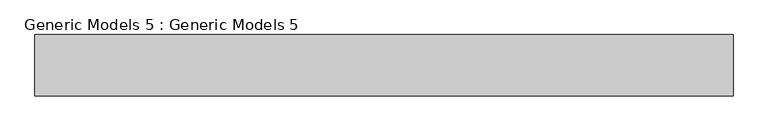
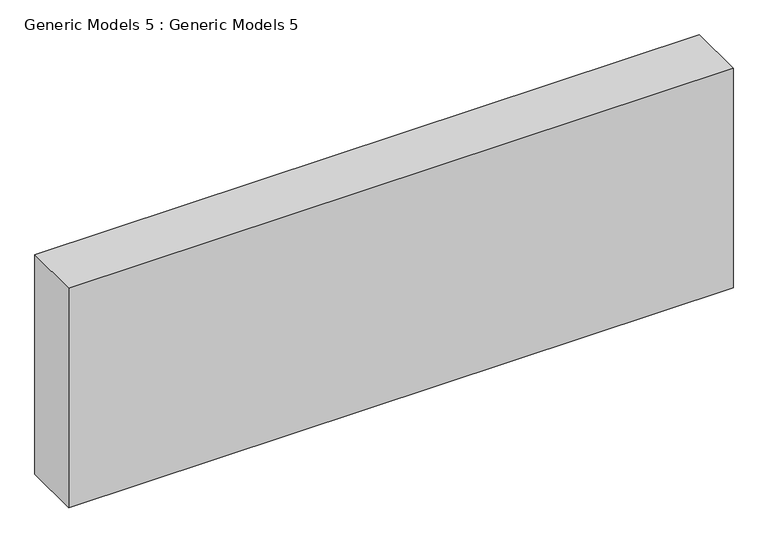
"""IFC4 building model written with IfcOpenShell, lengths in millimetres: proxy geometry, Generic Models 5 : Generic Models 5."""

from ifc_helpers import new_model, si_unit, frame, origin, place, context, project, spatial, polyline, outline, extrude, source, transform, mapped, element, save


def generic_models_5_generic_models_5_fbc28709(model_context):
    return source(origin(), model_context, "Body", "SweptSolid", [
        extrude(outline(polyline([(1172.1985746, -8793.5477377), (-2296.114408, -8793.5477377), (-2296.114408, -8488.7477377), (1172.1985746, -8488.7477377), (1172.1985746, -8793.5477377)])), frame((0.0, 0.0, 9776.2153024), z_axis=(0.0, 0.0, 1.0), x_axis=(1.0, 0.0, 0.0)), (0.0, 0.0, 1.0), 1210.3620819),
    ])


if __name__ == "__main__":
    model = new_model("IFC4")
    model_context = context("Model", 3, world=origin())
    ifc_project = project(units=[si_unit("LENGTHUNIT", "METRE", prefix="MILLI")], contexts=[model_context])
    site = spatial("IfcSite", under=ifc_project)
    building = spatial("IfcBuilding", under=site)
    placement = place(None, origin())
    generic_models_5_generic_models_5_shape = generic_models_5_generic_models_5_fbc28709(model_context)
    element("IfcBuildingElementProxy", 1, Name="Generic Models 5 : Generic Models 5", ObjectType="Generic Models 5 : Generic Models 5", at=placement, inside=building, context=model_context, shape_type="MappedRepresentation", body=[
        mapped(generic_models_5_generic_models_5_shape, transform((0.0, 0.0, 0.0), x_axis=(1.0, 0.0, 0.0), y_axis=(0.0, 1.0, 0.0), z_axis=(0.0, 0.0, 1.0))),
    ])
    save(model, "model.ifc")

# Revit data of these elements
# Element 1 (IfcBuildingElementProxy, "Generic Models 5 : Generic Models 5")
#   Materials on its faces: "Parking Stripe"
# Materials
#   "Parking Stripe": class "Paint", colour RGB 250 250 91, transparency 0, Cost = 0
